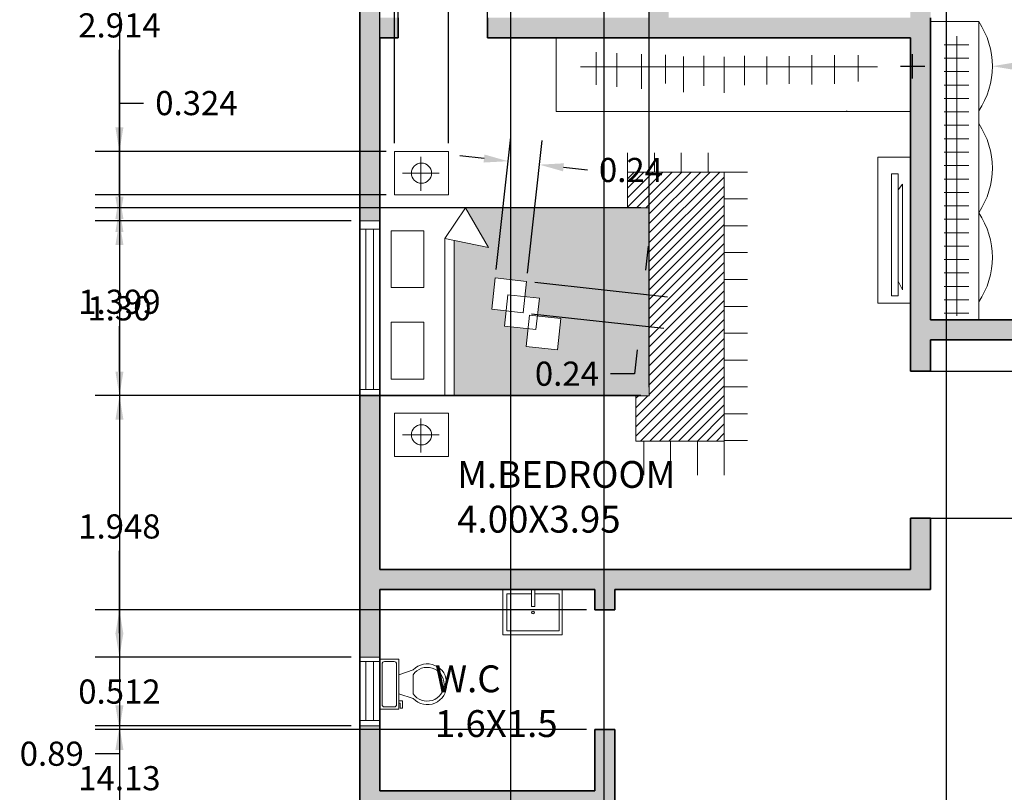
# Model space of a CAD drawing. Units: metres. Extents: x 36 to 56493, y 9 to 42849.
# Tile 3 of 5: x 56480.725 to 56488.056, y 42839.883 to 42845.639. Entities that reach past the tile are written whole.
import ezdxf

# ---------------------------------------------------------------- set-up
doc = ezdxf.new("R2010")
doc.units = ezdxf.units.M
doc.header["$MEASUREMENT"] = 0
for name, color, linetype, lineweight in [('A-ANNO-DIMS', 2, 'Continuous', 18), ('A-AREA-IDEN', 7, 'Continuous', 18), ('A-EQPM', 8, 'Continuous', 18), ('A-FLOR-CASE', 9, 'Continuous', 18), ('A-FLOR-FIXT', 8, 'Continuous', 18), ('A-FURN', 8, 'Continuous', 18), ('A-FURN-PATT', 252, 'Continuous', 13), ('A-GLAZ', 4, 'Continuous', 18), ('A-WALL', 7, 'Continuous', 35)]:
    doc.layers.add(name, color=color, linetype=linetype, lineweight=lineweight)
doc.layers.add('A-WALL-PATT', color=30, linetype='Continuous', lineweight=13, true_color=0xf26722)
doc.styles.get("Standard").update_dxf_attribs({"font": 'arial.ttf'})
doc.dimstyles.get("Standard").update_dxf_attribs({"dimtxt": 0.18, "dimasz": 0.18, "dimexe": 0.18, "dimexo": 0.0625, "dimgap": 0.09, "dimtad": 0, "dimtih": 1, "dimtoh": 1, "dimdec": 0, "dimzin": 0, "dimdsep": 46, "dimtxsty": 'Standard', "dimcen": 0.09, "dimadec": 0, "dimazin": 0, "dimtfac": 1, "dimtdec": 0, "dimtofl": 0, "dimtmove": 0, "dimatfit": 3, "dimfxl": 1, "dimtolj": 1, "dimtzin": 0, "dimarcsym": 0})

# ---------------------------------------------------------------- blocks, each defined once
blk = doc.blocks.new('*U2')
for p, q in [((9.5, -6), (9.5, -2)), ((-8, -8.5), (-8, -8)), ((-7, -8), (-7, -9.5)), ((-4, -8), (-6, -14)), ((4, -8), (6, -14)), ((-10, -8.5), (-8, -8.5)), ((-10, -9.5), (-10, -8.5)), ((-7, -9.5), (-10, -9.5)), ((4, -14), (-4, -14))]:
    blk.add_line(p, q)
blk.add_lwpolyline([(10.5, -8), (10.5, 0), (-10.5, 0), (-10.5, -8)], close=True)
for points in [[(-9.5, -2), (-9.5, -6)], [(8.5, -1), (-8.5, -1)], [(-8.5, -7), (8.5, -7)]]:
    blk.add_lwpolyline(points)
for centre, radius, start, end in [((-8.625, -1.875), 0.8839, 81.8699, 188.1301), ((8.625, -1.875), 0.8839, 351.8699, 98.1301), ((-8.625, -6.125), 0.8839, 171.869898, 278.1301), ((8.625, -6.125), 0.8839, 261.8699, 8.1301), ((-0.4772, -19.9188), 8.0953, 133.01722, 273.38), ((0.0374, -19.8731), 7.127, 124.50543, 269.7), ((-0.0373, -19.8731), 7.127, 270.3, 55.4946), ((0.4773, -19.9188), 8.0953, 266.62, 46.9828)]:
    blk.add_arc(centre, radius, start, end)
blk = doc.blocks.new('NIGHTSTAND-RECT')
for p, q in [((0.1969, 0.2836), (0.1969, 0.0315)), ((0.0601, 0.1624), (0.3337, 0.1624))]:
    blk.add_line(p, q)
blk.add_lwpolyline([(0.0004, 0.3243), (0.4019, 0.3243), (0.4019, 0.0004), (0.0004, 0.0004)], close=True)
blk.add_circle((0.2011, 0.1624), 0.0751)
blk = doc.blocks.new('CUSHION-SCATTER')
blk.add_lwpolyline([(0.2338, 0.0005), (0.2597, 0.2344), (0.0258, 0.2602), (0, 0.0263)], close=True)
blk = doc.blocks.new('*D18')
at = {"layer": 'A-ANNO-DIMS', "color": 0, "lineweight": -2, "transparency": 16777216}
for p, q in [((56483.1938, 42847.0533), (56481.2873, 42847.0533)), ((56481.4673, 42846.8733), (56481.4673, 42840.1703)), ((56481.4673, 42833.1033), (56481.4673, 42839.8063)), ((56483.1938, 42832.9233), (56481.2873, 42832.9233))]:
    blk.add_line(p, q, dxfattribs=at)
at = {"layer": 'A-ANNO-DIMS', "color": 0, "transparency": 16777216}
for points in [[(56481.4373, 42846.8733), (56481.4973, 42846.8733), (56481.4673, 42847.0533)], [(56481.4373, 42833.1033), (56481.4973, 42833.1033), (56481.4673, 42832.9233)]]:
    blk.add_solid(points, dxfattribs=at)
at = {"layer": 'Defpoints', "color": 0, "transparency": 16777216}
for p in [(56481.4673, 42847.0533), (56483.2563, 42847.0533), (56483.2563, 42832.9233)]:
    blk.add_point(p, dxfattribs=at)
at = {"layer": 'A-ANNO-DIMS', "color": 0, "transparency": 16777216, "insert": (56481.4673, 42839.9883), "char_height": 0.18, "attachment_point": 5}
blk.add_mtext('\\A1;14.13', dxfattribs=at)
blk = doc.blocks.new('*D25')
at = {"layer": 'A-ANNO-DIMS', "color": 0, "lineweight": -2, "transparency": 16777216}
for p, q in [((56483.5154, 42844.7198), (56483.5154, 42848.722)), ((56483.9169, 42844.7198), (56483.9169, 42848.722)), ((56483.3354, 42848.542), (56483.1554, 42848.542)), ((56484.0969, 42848.542), (56484.2769, 42848.542))]:
    blk.add_line(p, q, dxfattribs=at)
at = {"layer": 'A-ANNO-DIMS', "color": 0, "transparency": 16777216}
for points in [[(56483.3354, 42848.572), (56483.3354, 42848.512), (56483.5154, 42848.542)], [(56484.0969, 42848.572), (56484.0969, 42848.512), (56483.9169, 42848.542)]]:
    blk.add_solid(points, dxfattribs=at)
at = {"layer": 'Defpoints', "color": 0, "transparency": 16777216}
for p in [(56483.9169, 42848.542), (56483.5154, 42844.6573), (56483.9169, 42844.6573)]:
    blk.add_point(p, dxfattribs=at)
at = {"layer": 'A-ANNO-DIMS', "color": 0, "transparency": 16777216, "insert": (56484.6004, 42848.542), "char_height": 0.18, "attachment_point": 5}
blk.add_mtext('\\A1;0.40', dxfattribs=at)
blk = doc.blocks.new('*D26')
at = {"layer": 'A-ANNO-DIMS', "color": 0, "lineweight": -2, "transparency": 16777216}
for p, q in [((56481.4673, 42844.8373), (56481.4673, 42845.0173)), ((56481.4673, 42845.0173), (56481.6473, 42845.0173)), ((56483.4529, 42844.6573), (56481.2873, 42844.6573)), ((56483.4529, 42844.3334), (56481.2873, 42844.3334)), ((56481.4673, 42844.1534), (56481.4673, 42843.9734))]:
    blk.add_line(p, q, dxfattribs=at)
at = {"layer": 'A-ANNO-DIMS', "color": 0, "transparency": 16777216}
for points in [[(56481.4373, 42844.8373), (56481.4973, 42844.8373), (56481.4673, 42844.6573)], [(56481.4373, 42844.1534), (56481.4973, 42844.1534), (56481.4673, 42844.3334)]]:
    blk.add_solid(points, dxfattribs=at)
at = {"layer": 'Defpoints', "color": 0, "transparency": 16777216}
for p in [(56481.4673, 42844.6573), (56483.5154, 42844.6573), (56483.5154, 42844.3334)]:
    blk.add_point(p, dxfattribs=at)
at = {"layer": 'A-ANNO-DIMS', "color": 0, "transparency": 16777216, "insert": (56482.0406, 42845.0173), "char_height": 0.18, "attachment_point": 5}
blk.add_mtext('\\A1;0.324', dxfattribs=at)
blk = doc.blocks.new('*D29')
at = {"layer": 'A-ANNO-DIMS', "color": 0, "lineweight": -2, "transparency": 16777216}
for p, q in [((56484.2717, 42843.7773), (56484.3806, 42844.7633)), ((56484.5055, 42843.7515), (56484.6145, 42844.7375)), ((56484.1819, 42844.6042), (56484.003, 42844.624)), ((56484.7736, 42844.5388), (56484.9525, 42844.519))]:
    blk.add_line(p, q, dxfattribs=at)
at = {"layer": 'A-ANNO-DIMS', "color": 0, "transparency": 16777216}
for points in [[(56484.1852, 42844.634), (56484.1786, 42844.5744), (56484.3608, 42844.5844)], [(56484.7769, 42844.5686), (56484.7703, 42844.509), (56484.5947, 42844.5586)]]:
    blk.add_solid(points, dxfattribs=at)
at = {"layer": 'Defpoints', "color": 0, "transparency": 16777216}
for p in [(56484.5947, 42844.5586), (56484.2648, 42843.7152), (56484.4987, 42843.6894)]:
    blk.add_point(p, dxfattribs=at)
at = {"layer": 'A-ANNO-DIMS', "color": 0, "transparency": 16777216, "insert": (56485.2759, 42844.519), "char_height": 0.18, "attachment_point": 5}
blk.add_mtext('\\A1;0.24', dxfattribs=at)
blk = doc.blocks.new('*D30')
at = {"layer": 'A-ANNO-DIMS', "color": 0, "lineweight": -2, "transparency": 16777216}
for p, q in [((56485.3876, 42843.7722), (56485.4074, 42843.9511)), ((56484.5608, 42843.6825), (56485.5468, 42843.5735)), ((56484.5349, 42843.4486), (56485.5209, 42843.3397)), ((56485.3223, 42843.1805), (56485.3025, 42843.0016)), ((56485.3025, 42843.0016), (56485.1225, 42843.0016))]:
    blk.add_line(p, q, dxfattribs=at)
at = {"layer": 'A-ANNO-DIMS', "color": 0, "transparency": 16777216}
for points in [[(56485.3578, 42843.7755), (56485.4175, 42843.7689), (56485.3679, 42843.5933)], [(56485.2924, 42843.1838), (56485.3521, 42843.1772), (56485.342, 42843.3594)]]:
    blk.add_solid(points, dxfattribs=at)
at = {"layer": 'Defpoints', "color": 0, "transparency": 16777216}
for p in [(56484.4987, 42843.6894), (56484.4728, 42843.4555), (56485.342, 42843.3594)]:
    blk.add_point(p, dxfattribs=at)
at = {"layer": 'A-ANNO-DIMS', "color": 0, "transparency": 16777216, "insert": (56484.7991, 42843.0016), "char_height": 0.18, "attachment_point": 5}
blk.add_mtext('\\A1;0.24', dxfattribs=at)
blk = doc.blocks.new('*D35')
at = {"layer": 'A-ANNO-DIMS', "color": 0, "lineweight": -2, "transparency": 16777216}
for p, q in [((56484.382516, 42839.15308), (56484.382516, 42848.721953)), ((56485.07636, 42839.15308), (56485.07636, 42848.721953)), ((56484.202516, 42848.541953), (56484.022516, 42848.541953)), ((56485.25636, 42848.541953), (56485.43636, 42848.541953))]:
    blk.add_line(p, q, dxfattribs=at)
at = {"layer": 'A-ANNO-DIMS', "color": 0, "transparency": 16777216}
for points in [[(56484.202516, 42848.571953), (56484.202516, 42848.511953), (56484.382516, 42848.541953)], [(56485.25636, 42848.571953), (56485.25636, 42848.511953), (56485.07636, 42848.541953)]]:
    blk.add_solid(points, dxfattribs=at)
at = {"layer": 'Defpoints', "color": 0, "transparency": 16777216}
for p in [(56485.07636, 42848.541953), (56484.382516, 42839.09058), (56485.07636, 42839.09058)]:
    blk.add_point(p, dxfattribs=at)
at = {"layer": 'A-ANNO-DIMS', "color": 0, "transparency": 16777216, "insert": (56484.729438, 42848.541953), "char_height": 0.18, "attachment_point": 5}
blk.add_mtext('\\A1;0.69', dxfattribs=at)
blk = doc.blocks.new('*D48')
at = {"layer": 'A-ANNO-DIMS', "color": 0, "lineweight": -2, "transparency": 16777216}
for p, q in [((56483.1938, 42847.0533), (56481.2873, 42847.0533)), ((56481.4673, 42846.8733), (56481.4673, 42845.7781)), ((56481.4673, 42844.3191), (56481.4673, 42845.4143)), ((56483.1938, 42844.1391), (56481.2873, 42844.1391))]:
    blk.add_line(p, q, dxfattribs=at)
at = {"layer": 'A-ANNO-DIMS', "color": 0, "transparency": 16777216}
for points in [[(56481.4373, 42846.8733), (56481.4973, 42846.8733), (56481.4673, 42847.0533)], [(56481.4373, 42844.3191), (56481.4973, 42844.3191), (56481.4673, 42844.1391)]]:
    blk.add_solid(points, dxfattribs=at)
at = {"layer": 'Defpoints', "color": 0, "transparency": 16777216}
for p in [(56483.2563, 42847.0533), (56481.4673, 42844.1391), (56483.2563, 42844.1391)]:
    blk.add_point(p, dxfattribs=at)
at = {"layer": 'A-ANNO-DIMS', "color": 0, "transparency": 16777216, "insert": (56481.4673, 42845.5962), "char_height": 0.18, "attachment_point": 5}
blk.add_mtext('\\A1;2.914', dxfattribs=at)
blk = doc.blocks.new('*D49')
at = {"layer": 'A-ANNO-DIMS', "color": 0, "lineweight": -2, "transparency": 16777216}
for p, q in [((56483.1938, 42844.1391), (56481.2873, 42844.1391)), ((56481.4673, 42843.9591), (56481.4673, 42843.6705)), ((56481.4673, 42843.0179), (56481.4673, 42843.3065)), ((56483.1938, 42842.8379), (56481.2873, 42842.8379))]:
    blk.add_line(p, q, dxfattribs=at)
at = {"layer": 'A-ANNO-DIMS', "color": 0, "transparency": 16777216}
for points in [[(56481.4373, 42843.9591), (56481.4973, 42843.9591), (56481.4673, 42844.1391)], [(56481.4373, 42843.0179), (56481.4973, 42843.0179), (56481.4673, 42842.8379)]]:
    blk.add_solid(points, dxfattribs=at)
at = {"layer": 'Defpoints', "color": 0, "transparency": 16777216}
for p in [(56483.2563, 42844.1391), (56481.4673, 42842.8379), (56483.2563, 42842.8379)]:
    blk.add_point(p, dxfattribs=at)
at = {"layer": 'A-ANNO-DIMS', "color": 0, "transparency": 16777216, "insert": (56481.4673, 42843.4885), "char_height": 0.18, "attachment_point": 5}
blk.add_mtext('\\A1;1.30', dxfattribs=at)
blk = doc.blocks.new('*D50')
at = {"layer": 'A-ANNO-DIMS', "color": 0, "lineweight": -2, "transparency": 16777216}
for p, q in [((56483.1938, 42842.8379), (56481.2873, 42842.8379)), ((56481.4673, 42842.6579), (56481.4673, 42842.0457)), ((56481.4673, 42841.0698), (56481.4673, 42841.6819)), ((56483.1938, 42840.8898), (56481.2873, 42840.8898))]:
    blk.add_line(p, q, dxfattribs=at)
at = {"layer": 'A-ANNO-DIMS', "color": 0, "transparency": 16777216}
for points in [[(56481.4373, 42842.6579), (56481.4973, 42842.6579), (56481.4673, 42842.8379)], [(56481.4373, 42841.0698), (56481.4973, 42841.0698), (56481.4673, 42840.8898)]]:
    blk.add_solid(points, dxfattribs=at)
at = {"layer": 'Defpoints', "color": 0, "transparency": 16777216}
for p in [(56483.2563, 42842.8379), (56481.4673, 42840.8898), (56483.2563, 42840.8898)]:
    blk.add_point(p, dxfattribs=at)
at = {"layer": 'A-ANNO-DIMS', "color": 0, "transparency": 16777216, "insert": (56481.4673, 42841.8638), "char_height": 0.18, "attachment_point": 5}
blk.add_mtext('\\A1;1.948', dxfattribs=at)
blk = doc.blocks.new('*D51')
at = {"layer": 'A-ANNO-DIMS', "color": 0, "lineweight": -2, "transparency": 16777216}
for p, q in [((56481.4673, 42841.0698), (56481.4673, 42841.2498)), ((56483.1938, 42840.8898), (56481.2873, 42840.8898)), ((56483.1938, 42840.3779), (56481.2873, 42840.3779)), ((56481.4673, 42840.1979), (56481.4673, 42840.0179))]:
    blk.add_line(p, q, dxfattribs=at)
at = {"layer": 'A-ANNO-DIMS', "color": 0, "transparency": 16777216}
for points in [[(56481.4373, 42841.0698), (56481.4973, 42841.0698), (56481.4673, 42840.8898)], [(56481.4373, 42840.1979), (56481.4973, 42840.1979), (56481.4673, 42840.3779)]]:
    blk.add_solid(points, dxfattribs=at)
at = {"layer": 'Defpoints', "color": 0, "transparency": 16777216}
for p in [(56483.2563, 42840.8898), (56481.4673, 42840.3779), (56483.2563, 42840.3779)]:
    blk.add_point(p, dxfattribs=at)
at = {"layer": 'A-ANNO-DIMS', "color": 0, "transparency": 16777216, "insert": (56481.4673, 42840.6338), "char_height": 0.18, "attachment_point": 5}
blk.add_mtext('\\A1;0.512', dxfattribs=at)
blk = doc.blocks.new('*D52')
at = {"layer": 'A-ANNO-DIMS', "color": 0, "lineweight": -2, "transparency": 16777216}
for p, q in [((56483.1938, 42840.3779), (56481.2873, 42840.3779)), ((56481.4673, 42840.1979), (56481.4673, 42839.7207)), ((56481.4673, 42838.8797), (56481.4673, 42839.3569)), ((56483.1938, 42838.6997), (56481.2873, 42838.6997))]:
    blk.add_line(p, q, dxfattribs=at)
at = {"layer": 'A-ANNO-DIMS', "color": 0, "transparency": 16777216}
for points in [[(56481.4373, 42840.1979), (56481.4973, 42840.1979), (56481.4673, 42840.3779)], [(56481.4373, 42838.8797), (56481.4973, 42838.8797), (56481.4673, 42838.6997)]]:
    blk.add_solid(points, dxfattribs=at)
at = {"layer": 'Defpoints', "color": 0, "transparency": 16777216}
for p in [(56483.2563, 42840.3779), (56481.4673, 42838.6997), (56483.2563, 42838.6997)]:
    blk.add_point(p, dxfattribs=at)
at = {"layer": 'A-ANNO-DIMS', "color": 0, "transparency": 16777216, "insert": (56481.4673, 42839.5388), "char_height": 0.18, "attachment_point": 5}
blk.add_mtext('\\A1;1.678', dxfattribs=at)
blk = doc.blocks.new('*D56')
at = {"layer": 'A-ANNO-DIMS', "color": 0, "lineweight": -2, "transparency": 16777216}
for p, q in [((56483.4063, 42842.9004), (56483.4063, 42848.722)), ((56485.4125, 42842.9004), (56485.4125, 42848.722)), ((56483.5863, 42848.542), (56484.1015, 42848.542)), ((56485.2325, 42848.542), (56484.7173, 42848.542))]:
    blk.add_line(p, q, dxfattribs=at)
at = {"layer": 'A-ANNO-DIMS', "color": 0, "transparency": 16777216}
for points in [[(56483.5863, 42848.572), (56483.5863, 42848.512), (56483.4063, 42848.542)], [(56485.2325, 42848.572), (56485.2325, 42848.512), (56485.4125, 42848.542)]]:
    blk.add_solid(points, dxfattribs=at)
at = {"layer": 'Defpoints', "color": 0, "transparency": 16777216}
for p in [(56485.4125, 42848.542), (56483.4063, 42842.8379), (56485.4125, 42842.8379)]:
    blk.add_point(p, dxfattribs=at)
at = {"layer": 'A-ANNO-DIMS', "color": 0, "transparency": 16777216, "insert": (56484.4094, 42848.542), "char_height": 0.18, "attachment_point": 5}
blk.add_mtext('\\A1;2.01', dxfattribs=at)
blk = doc.blocks.new('*D57')
at = {"layer": 'A-ANNO-DIMS', "color": 0, "lineweight": -2, "transparency": 16777216}
for p, q in [((56485.35, 42844.2368), (56481.2873, 42844.2368)), ((56481.4673, 42844.0568), (56481.4673, 42843.7193)), ((56481.4673, 42843.0179), (56481.4673, 42843.3554)), ((56485.35, 42842.8379), (56481.2873, 42842.8379))]:
    blk.add_line(p, q, dxfattribs=at)
at = {"layer": 'A-ANNO-DIMS', "color": 0, "transparency": 16777216}
for points in [[(56481.4373, 42844.0568), (56481.4973, 42844.0568), (56481.4673, 42844.2368)], [(56481.4373, 42843.0179), (56481.4973, 42843.0179), (56481.4673, 42842.8379)]]:
    blk.add_solid(points, dxfattribs=at)
at = {"layer": 'Defpoints', "color": 0, "transparency": 16777216}
for p in [(56481.4673, 42844.2368), (56485.4125, 42844.2368), (56485.4125, 42842.8379)]:
    blk.add_point(p, dxfattribs=at)
at = {"layer": 'A-ANNO-DIMS', "color": 0, "transparency": 16777216, "insert": (56481.4673, 42843.5373), "char_height": 0.18, "attachment_point": 5}
blk.add_mtext('\\A1;1.399', dxfattribs=at)
blk = doc.blocks.new('*D62')
at = {"layer": 'A-ANNO-DIMS', "color": 0, "lineweight": -2, "transparency": 16777216}
for p, q in [((56483.5429, 42845.5658), (56483.5429, 42848.722)), ((56484.2087, 42845.5658), (56484.2087, 42848.722)), ((56483.3629, 42848.542), (56483.1829, 42848.542)), ((56484.3887, 42848.542), (56484.5687, 42848.542))]:
    blk.add_line(p, q, dxfattribs=at)
at = {"layer": 'A-ANNO-DIMS', "color": 0, "transparency": 16777216}
for points in [[(56483.3629, 42848.572), (56483.3629, 42848.512), (56483.5429, 42848.542)], [(56484.3887, 42848.572), (56484.3887, 42848.512), (56484.2087, 42848.542)]]:
    blk.add_solid(points, dxfattribs=at)
at = {"layer": 'Defpoints', "color": 0, "transparency": 16777216}
for p in [(56484.2087, 42848.542), (56483.5429, 42845.5033), (56484.2087, 42845.5033)]:
    blk.add_point(p, dxfattribs=at)
at = {"layer": 'A-ANNO-DIMS', "color": 0, "transparency": 16777216, "insert": (56483.8758, 42848.542), "char_height": 0.18, "attachment_point": 5}
blk.add_mtext('\\A1;0.67', dxfattribs=at)
blk = doc.blocks.new('*D64')
at = {"layer": 'A-ANNO-DIMS', "color": 0, "lineweight": -2, "transparency": 16777216}
for p, q in [((56487.4188, 42843.021), (56492.2108, 42843.021)), ((56492.0308, 42842.841), (56492.0308, 42842.6556)), ((56492.0308, 42842.1064), (56492.0308, 42842.2918)), ((56487.4188, 42841.9264), (56492.2108, 42841.9264))]:
    blk.add_line(p, q, dxfattribs=at)
at = {"layer": 'A-ANNO-DIMS', "color": 0, "transparency": 16777216}
for points in [[(56492.0008, 42842.841), (56492.0608, 42842.841), (56492.0308, 42843.021)], [(56492.0008, 42842.1064), (56492.0608, 42842.1064), (56492.0308, 42841.9264)]]:
    blk.add_solid(points, dxfattribs=at)
at = {"layer": 'Defpoints', "color": 0, "transparency": 16777216}
for p in [(56487.3563, 42843.021), (56487.3563, 42841.9264), (56492.0308, 42841.9264)]:
    blk.add_point(p, dxfattribs=at)
at = {"layer": 'A-ANNO-DIMS', "color": 0, "transparency": 16777216, "insert": (56492.0308, 42842.4737), "char_height": 0.18, "attachment_point": 5}
blk.add_mtext('\\A1;1.09', dxfattribs=at)
blk = doc.blocks.new('*D66')
at = {"layer": 'A-ANNO-DIMS', "color": 0, "lineweight": -2, "transparency": 16777216}
for p, q in [((56484.9438, 42841.2426), (56481.2873, 42841.2426)), ((56481.4673, 42841.0626), (56481.4673, 42840.531)), ((56484.9438, 42840.351), (56481.2873, 42840.351)), ((56481.4673, 42840.351), (56481.4673, 42840.171)), ((56481.4673, 42840.171), (56481.2873, 42840.171))]:
    blk.add_line(p, q, dxfattribs=at)
at = {"layer": 'A-ANNO-DIMS', "color": 0, "transparency": 16777216}
for points in [[(56481.4373, 42841.0626), (56481.4973, 42841.0626), (56481.4673, 42841.2426)], [(56481.4373, 42840.531), (56481.4973, 42840.531), (56481.4673, 42840.351)]]:
    blk.add_solid(points, dxfattribs=at)
at = {"layer": 'Defpoints', "color": 0, "transparency": 16777216}
for p in [(56485.0063, 42841.2426), (56481.4673, 42840.351), (56485.0063, 42840.351)]:
    blk.add_point(p, dxfattribs=at)
at = {"layer": 'A-ANNO-DIMS', "color": 0, "transparency": 16777216, "insert": (56480.9633, 42840.171), "char_height": 0.18, "attachment_point": 5}
blk.add_mtext('\\A1;0.89', dxfattribs=at)
blk = doc.blocks.new('*D67')
at = {"layer": 'A-ANNO-DIMS', "color": 0, "lineweight": -2, "transparency": 16777216}
for p, q in [((56487.626252, 42839.785791), (56487.626252, 42848.721953)), ((56488.392626, 42839.785791), (56488.392626, 42848.721953)), ((56487.446252, 42848.541953), (56487.266252, 42848.541953)), ((56488.572626, 42848.541953), (56488.752626, 42848.541953))]:
    blk.add_line(p, q, dxfattribs=at)
at = {"layer": 'A-ANNO-DIMS', "color": 0, "transparency": 16777216}
for points in [[(56487.446252, 42848.571953), (56487.446252, 42848.511953), (56487.626252, 42848.541953)], [(56488.572626, 42848.571953), (56488.572626, 42848.511953), (56488.392626, 42848.541953)]]:
    blk.add_solid(points, dxfattribs=at)
at = {"layer": 'Defpoints', "color": 0, "transparency": 16777216}
for p in [(56488.392626, 42848.541953), (56487.626252, 42839.723291), (56488.392626, 42839.723291)]:
    blk.add_point(p, dxfattribs=at)
at = {"layer": 'A-ANNO-DIMS', "color": 0, "transparency": 16777216, "insert": (56488.009439, 42848.541953), "char_height": 0.18, "attachment_point": 5}
blk.add_mtext('\\A1;0.77', dxfattribs=at)
blk = doc.blocks.new('*D71')
at = {"layer": 'A-ANNO-DIMS', "color": 0, "lineweight": -2, "transparency": 16777216}
for p, q in [((56487.3732, 42845.2016), (56487.3732, 42845.3816)), ((56487.2832, 42845.2916), (56487.4632, 42845.2916)), ((56488.3266, 42845.2922), (56488.1466, 42845.2921))]:
    blk.add_line(p, q, dxfattribs=at)
at = {"layer": 'A-ANNO-DIMS', "color": 0, "transparency": 16777216}
blk.add_solid([(56488.1466, 42845.3221), (56488.1466, 42845.2621), (56487.9666, 42845.292)], dxfattribs=at)
at = {"layer": 'Defpoints', "color": 0, "transparency": 16777216}
for p in [(56487.3732, 42845.2916), (56487.9666, 42845.292)]:
    blk.add_point(p, dxfattribs=at)
at = {"layer": 'A-ANNO-DIMS', "color": 0, "transparency": 16777216, "insert": (56488.9337, 42845.2922), "char_height": 0.18, "attachment_point": 5}
blk.add_mtext('\\A1;4X R0.59', dxfattribs=at)

msp = doc.modelspace()

# ---------------------------------------------------------------- hatches: boundary and pattern name
at = {"layer": 'A-FURN-PATT'}
h = msp.add_hatch(dxfattribs=at)
h.set_pattern_fill('ANSI31', color=256, scale=0.4)
h.set_pattern_definition([(45, (0, 0), (-0.03535533906, 0.03535533906), [])])
h.paths.add_polyline_path([(56485.9707, 42844.5032), (56485.251, 42844.5032), (56485.251, 42844.2368), (56485.4125, 42844.2368), (56485.4125, 42842.8378), (56485.3123, 42842.8378), (56485.3123, 42842.4991), (56485.9707, 42842.4991), (56485.9707, 42842.5032)])
h = msp.add_hatch(color=256, dxfattribs=at)
h.dxf.hatch_style = 1
h.paths.add_polyline_path([(56485.4125, 42844.2368), (56484.0449, 42844.2368), (56484.2157, 42843.9411), (56483.9591, 42843.9953), (56483.9591, 42842.8378), (56485.4125, 42842.8378)])
h.paths.add_polyline_path([(56484.7544, 42843.4123), (56484.7285, 42843.1785), (56484.4947, 42843.2043), (56484.5093, 42843.3365), (56484.3343, 42843.3558), (56484.3469, 42843.4694), (56484.239, 42843.4813), (56484.2648, 42843.7152), (56484.4987, 42843.6894), (56484.4861, 42843.5758), (56484.594, 42843.5638), (56484.5794, 42843.4317)], flags=16)
at = {"layer": 'A-WALL-PATT'}
h = msp.add_hatch(color=256, dxfattribs=at)
h.dxf.hatch_style = 1
edge = h.paths.add_edge_path()
edge.add_line((56483.5429, 42845.6533), (56483.4063, 42845.6533))
edge.add_line((56483.4063, 42845.6533), (56483.4063, 42846.9033))
edge.add_line((56483.4063, 42846.9033), (56483.63, 42846.9033))
edge.add_ellipse((56483.6664, 42846.7323), major_axis=(0.2141, -0.003), ratio=0.809245, start_angle=94.07135, end_angle=102.818, ccw=False)
edge.add_line((56483.6565, 42846.9062), (56483.6565, 42846.9056))
edge.add_line((56483.6565, 42846.9056), (56483.6615, 42846.9056))
edge.add_ellipse((56483.6664, 42846.7323), major_axis=(0.2141, -0.003), ratio=0.809245, start_angle=90, end_angle=92.42655, ccw=False)
edge.add_line((56483.6812, 42846.9058), (56483.6812, 42846.9052))
edge.add_ellipse((56483.6664, 42846.7323), major_axis=(0.2141, -0.003), ratio=0.809245, start_angle=79.57494, end_angle=85.92601, ccw=False)
edge.add_line((56483.7048, 42846.9033), (56484.1418, 42846.9033))
edge.add_line((56484.1418, 42846.9033), (56484.1418, 42847.0533))
edge.add_line((56484.1418, 42847.0533), (56483.2563, 42847.0533))
edge.add_line((56483.2563, 42847.0533), (56483.2563, 42844.1391))
edge.add_line((56483.2563, 42844.1391), (56483.4063, 42844.1391))
edge.add_line((56483.4063, 42844.1391), (56483.4063, 42844.2368))
edge.add_line((56483.4063, 42844.2368), (56483.4063, 42845.5033))
edge.add_line((56483.4063, 42845.5033), (56483.5429, 42845.5033))
edge.add_line((56483.5429, 42845.5033), (56483.5429, 42845.6533))
edge = h.paths.add_edge_path(flags=0)
edge.add_line((56488.6347, 42847.0533), (56486.6826, 42847.0533))
edge.add_line((56486.6826, 42847.0533), (56486.6826, 42846.9033))
edge.add_line((56486.6826, 42846.9033), (56486.9892, 42846.9033))
edge.add_ellipse((56487.0257, 42846.7323), major_axis=(0.2141, -0.003), ratio=0.809245, start_angle=94.07135, end_angle=102.818, ccw=False)
edge.add_line((56487.0157, 42846.9062), (56487.0157, 42846.9056))
edge.add_line((56487.0157, 42846.9056), (56487.0207, 42846.9056))
edge.add_ellipse((56487.0257, 42846.7323), major_axis=(0.2141, -0.003), ratio=0.809245, start_angle=90, end_angle=92.42655, ccw=False)
edge.add_line((56487.0404, 42846.9058), (56487.0404, 42846.9052))
edge.add_ellipse((56487.0257, 42846.7323), major_axis=(0.2141, -0.003), ratio=0.809245, start_angle=79.57494, end_angle=85.92601, ccw=False)
edge.add_line((56487.064, 42846.9033), (56487.3563, 42846.9033))
edge.add_line((56487.3563, 42846.9033), (56487.3563, 42846.6728))
edge.add_line((56487.3563, 42846.6728), (56487.5063, 42846.6728))
edge.add_line((56487.5063, 42846.6728), (56487.5063, 42846.9033))
edge.add_line((56487.5063, 42846.9033), (56488.6347, 42846.9033))
edge.add_line((56488.6347, 42846.9033), (56488.6347, 42847.0533))
h.paths.add_polyline_path([(56486.2245, 42847.0533), (56484.665, 42847.0533), (56484.665, 42846.9033), (56485.4063, 42846.9033), (56485.4063, 42845.6533), (56484.2087, 42845.6533), (56484.2087, 42845.5033), (56487.3563, 42845.5033), (56487.3563, 42844.954), (56487.3563, 42843.021), (56487.5063, 42843.021), (56487.5063, 42843.2533), (56489.9401, 42843.2533), (56489.9401, 42843.4033), (56487.5063, 42843.4033), (56487.5063, 42845.6238), (56487.5063, 42845.6533), (56487.5063, 42845.9366), (56487.3563, 42845.9366), (56487.3563, 42845.6533), (56485.5563, 42845.6533), (56485.5563, 42846.9033), (56486.2245, 42846.9033)])
h.paths.add_polyline_path([(56491.1563, 42847.0533), (56489.9198, 42847.0533), (56489.9198, 42846.9033), (56489.9717, 42846.9033), (56491.0063, 42846.9033), (56491.0063, 42845.887), (56491.1563, 42845.887)])
h.paths.add_polyline_path([(56491.1563, 42844.3264), (56491.0063, 42844.3264), (56491.0063, 42843.4033), (56490.7805, 42843.4033), (56490.7805, 42843.2533), (56491.0063, 42843.2533), (56491.0063, 42839.8733), (56488.3926, 42839.8733), (56488.3926, 42839.7233), (56491.0063, 42839.7233), (56491.0063, 42836.1233), (56487.6263, 42836.1233), (56487.6263, 42839.0009), (56487.4763, 42839.0009), (56487.4763, 42836.1233), (56486.4863, 42836.1233), (56486.4863, 42835.9733), (56487.4763, 42835.9733), (56487.8849, 42835.9733), (56487.8849, 42832.9233), (56487.8913, 42832.9233), (56488.0349, 42832.9233), (56488.0349, 42833.0733), (56488.0349, 42835.9733), (56491.0063, 42835.9733), (56491.0063, 42833.0733), (56491.0063, 42832.9233), (56491.1563, 42832.9233), (56491.1563, 42835.9733)])
h.paths.add_polyline_path([(56483.4063, 42842.8378), (56483.2563, 42842.8378), (56483.2563, 42841.5433), (56483.2563, 42840.8898), (56483.4063, 42840.8898), (56483.4063, 42841.3933), (56485.0063, 42841.3933), (56485.0063, 42841.2426), (56485.1563, 42841.2426), (56485.1563, 42841.3933), (56487.3563, 42841.3933), (56487.5063, 42841.3933), (56487.5063, 42841.9264), (56487.3563, 42841.9264), (56487.3563, 42841.5433), (56483.4063, 42841.5433)])
h.paths.add_polyline_path([(56485.1563, 42840.351), (56485.0063, 42840.351), (56485.0063, 42839.8933), (56483.4063, 42839.8933), (56483.4063, 42840.3779), (56483.2563, 42840.3779), (56483.2563, 42839.8933), (56483.2563, 42838.6997), (56483.4063, 42838.6997), (56483.4063, 42839.7433), (56485.1563, 42839.7433)])
h.paths.add_polyline_path([(56483.4063, 42836.7612), (56483.2563, 42836.7612), (56483.2563, 42835.6733), (56483.2563, 42834.2533), (56483.2563, 42832.9233), (56485.9871, 42832.9233), (56485.9871, 42833.0733), (56483.4063, 42833.0733), (56483.4063, 42834.2533), (56483.4063, 42835.5233), (56485.4763, 42835.5233), (56485.9871, 42835.5233), (56485.9871, 42835.6733), (56485.6263, 42835.6733), (56483.4063, 42835.6733)])

# ---------------------------------------------------------------- linework, layer by layer
at = {"layer": 'A-EQPM'}
for p, q in [((56487.2656, 42844.3721), (56487.2982, 42844.4134)), ((56487.2982, 42844.4134), (56487.2982, 42843.6269)), ((56487.2982, 42843.6269), (56487.2656, 42843.6914))]:
    msp.add_line(p, q, dxfattribs=at)
for points in [[(56487.3563, 42844.6153), (56487.1148, 42844.6153), (56487.1148, 42843.5266), (56487.3563, 42843.5266)], [(56487.2155, 42844.491), (56487.2656, 42844.491), (56487.2656, 42843.5806), (56487.2155, 42843.5806)]]:
    msp.add_lwpolyline(points, close=True, dxfattribs=at)
at = {"layer": 'A-FLOR-CASE'}
for p, q in [((56487.7022, 42845.5161), (56487.7022, 42843.432)), ((56485.0181, 42845.3969), (56485.0181, 42845.1544)), ((56485.1708, 42845.389), (56485.1708, 42845.1388)), ((56485.3549, 42845.3812), (56485.3549, 42845.1231)), ((56487.6078, 42845.4517), (56487.7921, 42845.4517)), ((56485.5328, 42845.3764), (56485.5328, 42845.1624)), ((56485.6682, 42845.3641), (56485.6682, 42845.0985)), ((56485.8184, 42845.369), (56485.8184, 42845.1452)), ((56485.9711, 42845.3616), (56485.9711, 42845.0936)), ((56486.1213, 42845.369), (56486.1213, 42845.1501)), ((56486.2888, 42845.3641), (56486.2888, 42845.155)), ((56486.4538, 42845.3666), (56486.4538, 42845.16)), ((56486.6237, 42845.3739), (56486.6237, 42845.155)), ((56486.7911, 42845.3739), (56486.7911, 42845.16)), ((56486.9684, 42845.3739), (56486.9684, 42845.1772)), ((56487.6078, 42845.3517), (56487.7921, 42845.3517)), ((56484.9015, 42845.2873), (56487.1122, 42845.2873)), ((56487.6078, 42845.2517), (56487.7921, 42845.2517)), ((56487.6078, 42845.1517), (56487.7921, 42845.1517)), ((56487.6078, 42845.0517), (56487.7921, 42845.0517)), ((56487.6078, 42844.9517), (56487.7921, 42844.9517)), ((56487.6078, 42844.8517), (56487.7921, 42844.8517)), ((56487.6078, 42844.7517), (56487.7921, 42844.7517)), ((56487.6078, 42844.6517), (56487.7921, 42844.6517)), ((56487.6078, 42844.5517), (56487.7921, 42844.5517)), ((56487.6078, 42844.4517), (56487.7921, 42844.4517)), ((56487.6078, 42844.3517), (56487.7921, 42844.3517)), ((56487.6078, 42844.2517), (56487.7921, 42844.2517)), ((56487.6078, 42844.1517), (56487.7921, 42844.1517)), ((56487.6078, 42844.0517), (56487.7921, 42844.0517)), ((56487.6078, 42843.9517), (56487.7921, 42843.9517)), ((56487.6078, 42843.8517), (56487.7921, 42843.8517)), ((56487.6078, 42843.7517), (56487.7921, 42843.7517)), ((56487.6078, 42843.6517), (56487.7921, 42843.6517)), ((56487.6078, 42843.5517), (56487.7921, 42843.5517)), ((56487.6078, 42843.4517), (56487.7921, 42843.4517))]:
    msp.add_line(p, q, dxfattribs=at)
for points in [[(56487.5063, 42845.6238), (56487.8649, 42845.6238), (56487.8649, 42843.4033), (56487.5063, 42843.4033)], [(56484.7179, 42845.5033), (56487.3563, 42845.5033), (56487.3563, 42844.954), (56484.7179, 42844.954)]]:
    msp.add_lwpolyline(points, close=True, dxfattribs=at)
for centre, start, end in [((56487.3732, 42845.2916), 325.957, 34.043), ((56487.3732, 42845.2916), 214.043, 214.67165), ((56487.3732, 42844.5327), 325.957, 34.043), ((56487.3732, 42843.8683), 325.957, 34.043)]:
    msp.add_arc(centre, 0.5934, start, end, dxfattribs=at)
at = {"layer": 'A-FLOR-FIXT'}
for points in [[(56484.3211, 42841.3933), (56484.763, 42841.3933), (56484.763, 42841.0566), (56484.3211, 42841.0566)], [(56484.5611, 42841.3933), (56484.5343, 42841.3933), (56484.5343, 42841.2671), (56484.5611, 42841.2671)]]:
    msp.add_lwpolyline(points, close=True, dxfattribs=at)
msp.add_lwpolyline([(56484.5611, 42841.3616), (56484.7405, 42841.3616), (56484.7405, 42841.0852), (56484.353, 42841.0852), (56484.353, 42841.3616), (56484.5343, 42841.3616)], dxfattribs=at)
msp.add_circle((56484.5468, 42841.2234), 0.0102, dxfattribs=at)
at = {"layer": 'A-FURN'}
for p, q in [((56485.251, 42844.5032), (56485.251, 42844.6479)), ((56485.451, 42844.5032), (56485.451, 42844.6479)), ((56485.651, 42844.5032), (56485.651, 42844.6479)), ((56485.851, 42844.5032), (56485.851, 42844.6479)), ((56485.251, 42844.2368), (56485.251, 42844.5032)), ((56485.251, 42844.5032), (56485.9707, 42844.5032)), ((56485.9707, 42844.5032), (56485.9707, 42842.4991)), ((56485.9707, 42844.5032), (56486.1431, 42844.5032)), ((56485.9707, 42844.3032), (56486.1431, 42844.3032)), ((56483.8908, 42844.0098), (56484.0449, 42844.2368)), ((56484.0449, 42844.2368), (56484.2157, 42843.9411)), ((56485.9707, 42844.1032), (56486.1431, 42844.1032)), ((56483.8908, 42842.8378), (56483.8908, 42844.0098)), ((56484.2157, 42843.9411), (56483.8908, 42844.0098)), ((56483.9591, 42843.9953), (56483.9591, 42842.8378)), ((56485.9707, 42843.9032), (56486.1431, 42843.9032)), ((56485.9707, 42843.7032), (56486.1431, 42843.7032)), ((56485.9707, 42843.5032), (56486.1431, 42843.5032)), ((56485.9707, 42843.3032), (56486.1431, 42843.3032)), ((56485.9707, 42843.1032), (56486.1431, 42843.1032)), ((56485.9707, 42842.9032), (56486.1431, 42842.9032)), ((56485.3123, 42842.4991), (56485.3123, 42842.8378)), ((56485.9707, 42842.7032), (56486.1431, 42842.7032)), ((56485.9707, 42842.4991), (56485.3123, 42842.4991)), ((56485.3707, 42842.4991), (56485.3707, 42842.2469)), ((56485.5707, 42842.4991), (56485.5707, 42842.2469)), ((56485.7707, 42842.4991), (56485.7707, 42842.2469)), ((56485.9707, 42842.5032), (56486.1431, 42842.5032)), ((56485.9707, 42842.4991), (56485.9707, 42842.2469))]:
    msp.add_line(p, q, dxfattribs=at)
for points in [[(56483.4063, 42842.8378), (56485.4125, 42842.8378), (56485.4125, 42844.2368), (56483.4063, 42844.2368)], [(56483.4914, 42844.0669), (56483.7341, 42844.0669), (56483.7341, 42843.6438), (56483.4914, 42843.6438)], [(56483.4914, 42843.3848), (56483.7341, 42843.3848), (56483.7341, 42842.9616), (56483.4914, 42842.9616)]]:
    msp.add_lwpolyline(points, close=True, dxfattribs=at)
at = {"layer": 'A-GLAZ'}
for p, q in [((56483.2563, 42844.1391), (56483.4063, 42844.1391)), ((56483.2563, 42844.0789), (56483.4063, 42844.0789)), ((56483.3022, 42844.0789), (56483.3022, 42842.8849)), ((56483.3585, 42844.0789), (56483.3585, 42842.8849)), ((56483.2563, 42842.8849), (56483.4063, 42842.8849)), ((56483.2563, 42842.8378), (56483.4063, 42842.8378)), ((56483.2563, 42840.8898), (56483.4063, 42840.8898)), ((56483.2563, 42840.8589), (56483.4063, 42840.8589)), ((56483.3018, 42840.8589), (56483.3018, 42840.418)), ((56483.3594, 42840.8589), (56483.3594, 42840.418)), ((56483.2563, 42840.418), (56483.4063, 42840.418)), ((56483.2563, 42840.3779), (56483.4063, 42840.3779))]:
    msp.add_line(p, q, dxfattribs=at)
at = {"layer": 'A-WALL'}
for p, q in [((56483.2563, 42834.2533), (56483.2563, 42847.0533)), ((56483.5429, 42845.6533), (56483.5429, 42845.5033)), ((56484.2087, 42845.6533), (56484.2087, 42845.5033)), ((56487.5063, 42843.4033), (56487.5063, 42845.6533)), ((56483.2563, 42845.5033), (56483.2563, 42841.5433)), ((56483.4063, 42845.5033), (56483.4063, 42841.5433)), ((56483.5429, 42845.5033), (56483.4063, 42845.5033)), ((56483.5429, 42845.5033), (56483.4063, 42845.5033)), ((56485.4063, 42845.5033), (56484.2087, 42845.5033)), ((56487.3563, 42845.5033), (56484.2087, 42845.5033)), ((56487.3563, 42843.021), (56487.3563, 42845.5033)), ((56489.9401, 42843.4033), (56487.5063, 42843.4033)), ((56487.3563, 42843.021), (56487.3563, 42843.2533)), ((56487.5063, 42843.021), (56487.5063, 42843.2533)), ((56489.9401, 42843.2533), (56487.5063, 42843.2533)), ((56487.3563, 42843.021), (56487.5063, 42843.021)), ((56487.3563, 42841.5433), (56487.3563, 42841.9264)), ((56487.3563, 42841.9264), (56487.5063, 42841.9264)), ((56487.3563, 42841.5433), (56487.3563, 42841.9264)), ((56487.5063, 42841.3933), (56487.5063, 42841.9264)), ((56483.4063, 42841.5433), (56487.3563, 42841.5433)), ((56483.2563, 42841.3933), (56483.2563, 42839.8933)), ((56483.4063, 42841.3933), (56485.0063, 42841.3933)), ((56483.4063, 42841.3933), (56483.4063, 42839.8933)), ((56485.0063, 42841.2426), (56485.0063, 42841.3933)), ((56485.1563, 42841.3933), (56487.3563, 42841.3933)), ((56485.1563, 42841.2426), (56485.1563, 42841.3933)), ((56487.3563, 42841.3933), (56487.5063, 42841.3933)), ((56485.0063, 42841.2426), (56485.1563, 42841.2426)), ((56485.0063, 42839.8933), (56485.0063, 42840.351)), ((56485.0063, 42840.351), (56485.1563, 42840.351)), ((56485.1563, 42839.7433), (56485.1563, 42840.351)), ((56483.4063, 42839.8933), (56485.0063, 42839.8933))]:
    msp.add_line(p, q, dxfattribs=at)

# ---------------------------------------------------------------- block references
at = {"layer": 'A-FLOR-FIXT', "xscale": 0.01774095366731, "yscale": 0.01774095366731, "zscale": 0.01774095366731, "rotation": 90}
msp.add_blockref('*U2', (56483.4063, 42840.6882), dxfattribs=at)
at = {"layer": 'A-FURN'}
for name, p in [('NIGHTSTAND-RECT', (56483.515, 42844.333)), ('CUSHION-SCATTER', (56484.239, 42843.455)), ('CUSHION-SCATTER', (56484.3343, 42843.3295)), ('CUSHION-SCATTER', (56484.4947, 42843.178)), ('NIGHTSTAND-RECT', (56483.515, 42842.384))]:
    msp.add_blockref(name, p, dxfattribs=at)

# ---------------------------------------------------------------- texts
at = {"layer": 'A-AREA-IDEN', "char_height": 0.2, "attachment_point": 1}
for s, insert in [('M.BEDROOM\\P4.00X3.95', (56483.9821, 42842.3512)), ('W.C\\P1.6X1.5', (56483.8162, 42840.8287))]:
    msp.add_mtext_dynamic_manual_height_columns(s, width=0.817901, gutter_width=1, heights=[0], dxfattribs=dict(at, insert=insert))

# ---------------------------------------------------------------- dimensions: what is measured, and where the dimension line sits
at = {"layer": 'A-ANNO-DIMS'}
for base, p1, p2, picture, middle in [((56483.9169, 42848.542), (56483.5154, 42844.6573), (56483.9169, 42844.6573), '*D25', (56484.6004, 42848.542)), ((56484.2087, 42848.542), (56483.5429, 42845.5033), (56484.2087, 42845.5033), '*D62', (56483.8758, 42848.542)), ((56485.4125, 42848.542), (56483.4063, 42842.8378), (56485.4125, 42842.8378), '*D56', (56484.4094, 42848.542)), ((56485.0764, 42848.542), (56484.3825, 42839.0906), (56485.0764, 42839.0906), '*D35', (56484.7294, 42848.542)), ((56488.3926, 42848.542), (56487.6263, 42839.7233), (56488.3926, 42839.7233), '*D67', (56488.0094, 42848.542))]:
    dim = msp.add_linear_dim(base=base, p1=p1, p2=p2, dimstyle='Standard', override={"dimdec": 2, "dimlfac": 1, "dimrnd": 0, "dimzin": 0, "dimdsep": 46, "dimlunit": 2}, dxfattribs=at)
    dim.commit()
    dim.dimension.update_dxf_attribs({"geometry": picture, "text_midpoint": middle})
for base, p1, p2, angle, override, picture, middle in [((56481.4673, 42847.0533), (56483.2563, 42832.9233), (56483.2563, 42847.0533), 90, {"dimdec": 2, "dimlfac": 1, "dimrnd": 0, "dimzin": 0, "dimdsep": 46, "dimlunit": 2}, '*D18', (56481.4673, 42839.9883)), ((56481.4673, 42844.1391), (56483.2563, 42847.0533), (56483.2563, 42844.1391), 90, {"dimdec": 3, "dimlfac": 1, "dimrnd": 0, "dimzin": 0, "dimdsep": 46, "dimlunit": 2}, '*D48', (56481.4673, 42845.5962)), ((56481.4673, 42844.6573), (56483.5154, 42844.3334), (56483.5154, 42844.6573), 90, {"dimdec": 3, "dimlfac": 1, "dimrnd": 0, "dimzin": 0, "dimdsep": 46, "dimlunit": 2}, '*D26', (56482.0406, 42845.0173)), ((56484.5947, 42844.5586), (56484.2648, 42843.7152), (56484.4987, 42843.6894), 353.69449, {"dimdec": 2, "dimlfac": 1, "dimrnd": 0, "dimzin": 0, "dimdsep": 46, "dimlunit": 2}, '*D29', (56485.2759, 42844.519)), ((56481.4673, 42844.2368), (56485.4125, 42842.8378), (56485.4125, 42844.2368), 90, {"dimdec": 3, "dimlfac": 1, "dimrnd": 0, "dimzin": 0, "dimdsep": 46, "dimlunit": 2}, '*D57', (56481.4673, 42843.5373)), ((56481.4673, 42842.8378), (56483.2563, 42844.1391), (56483.2563, 42842.8378), 90, {"dimdec": 2, "dimlfac": 1, "dimrnd": 0, "dimzin": 0, "dimdsep": 46, "dimlunit": 2}, '*D49', (56481.4673, 42843.4885)), ((56485.342, 42843.3594), (56484.4987, 42843.6894), (56484.4728, 42843.4555), 263.69449, {"dimdec": 2, "dimlfac": 1, "dimrnd": 0, "dimzin": 0, "dimdsep": 46, "dimlunit": 2}, '*D30', (56484.7991, 42843.0016)), ((56492.0308, 42841.9264), (56487.3563, 42843.021), (56487.3563, 42841.9264), 90, {"dimdec": 2, "dimlfac": 1, "dimrnd": 0, "dimzin": 0, "dimdsep": 46, "dimlunit": 2}, '*D64', (56492.0308, 42842.4737)), ((56481.4673, 42840.8898), (56483.2563, 42842.8378), (56483.2563, 42840.8898), 90, {"dimdec": 3, "dimlfac": 1, "dimrnd": 0, "dimzin": 0, "dimdsep": 46, "dimlunit": 2}, '*D50', (56481.4673, 42841.8638)), ((56481.4673, 42840.351), (56485.0063, 42841.2426), (56485.0063, 42840.351), 90, {"dimdec": 2, "dimlfac": 1, "dimrnd": 0, "dimzin": 0, "dimdsep": 46, "dimlunit": 2}, '*D66', (56480.9633, 42840.171)), ((56481.4673, 42840.3779), (56483.2563, 42840.8898), (56483.2563, 42840.3779), 90, {"dimdec": 3, "dimlfac": 1, "dimrnd": 0, "dimzin": 0, "dimdsep": 46, "dimlunit": 2}, '*D51', (56481.4673, 42840.6338)), ((56481.4673, 42838.6997), (56483.2563, 42840.3779), (56483.2563, 42838.6997), 90, {"dimdec": 3, "dimlfac": 1, "dimrnd": 0, "dimzin": 0, "dimdsep": 46, "dimlunit": 2}, '*D52', (56481.4673, 42839.5388))]:
    dim = msp.add_linear_dim(base=base, p1=p1, p2=p2, angle=angle, dimstyle='Standard', override=override, dxfattribs=at)
    dim.commit()
    dim.dimension.update_dxf_attribs({"geometry": picture, "text_midpoint": middle})
dim = msp.add_radius_dim(center=(56487.3732, 42845.2916), mpoint=(56487.9666, 42845.292), text='4X <>', dimstyle='Standard', override={"dimdec": 2, "dimlfac": 1, "dimrnd": 0, "dimzin": 0, "dimdsep": 46, "dimlunit": 2}, dxfattribs=at)
dim.commit()
dim.dimension.update_dxf_attribs({"geometry": '*D71', "text_midpoint": (56488.9337, 42845.2922)})

doc.saveas('drawing.dxf')
